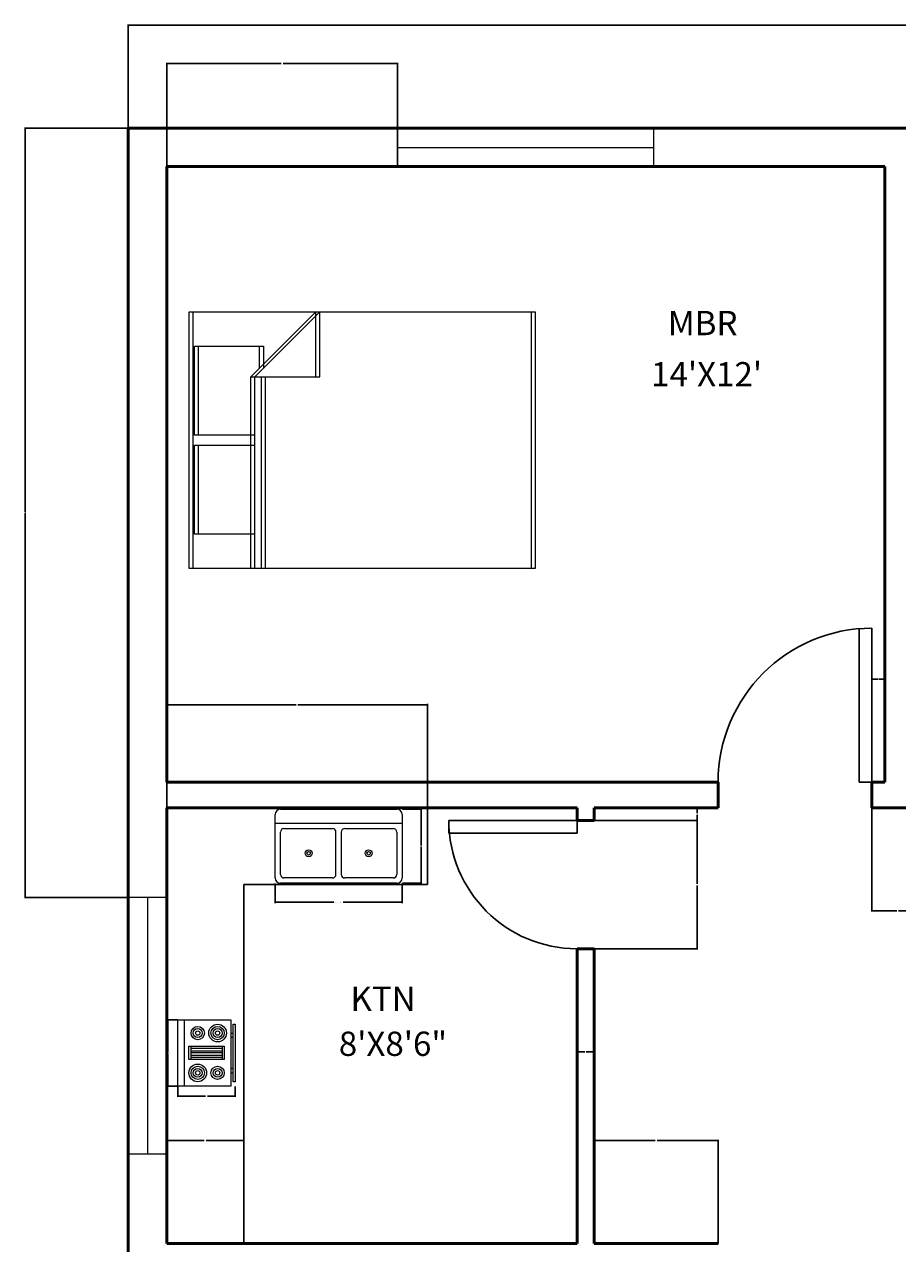
# Model space of a CAD drawing. Units: inches. Extents: x 66 to 499, y 601 to 1111.
# Tile 3 of 4: x 66 to 271, y 826 to 1111. Entities that reach past the tile are written whole.
import ezdxf

# ---------------------------------------------------------------- set-up
doc = ezdxf.new("R2010")
doc.units = ezdxf.units.IN
for name, color, linetype, lineweight in [('A-ANNO-DIMS', 2, 'Continuous', 18), ('A-AREA-IDEN', 7, 'Continuous', 18), ('A-DOOR', 3, 'Continuous', 25), ('A-EQPM', 8, 'Continuous', 18), ('A-FLOR-CASE', 9, 'Continuous', 25), ('A-FLOR-FIXT', 9, 'Continuous', 18), ('A-FURN', 8, 'Continuous', 18), ('A-GLAZ', 4, 'Continuous', 18), ('A-WALL', 7, 'Continuous', 50)]:
    doc.layers.add(name, color=color, linetype=linetype, lineweight=lineweight)
doc.styles.get("Standard").update_dxf_attribs({"font": 'arial.ttf'})
doc.dimstyles.get("Standard").update_dxf_attribs({"dimtxt": 0.18, "dimasz": 0.18, "dimexe": 0.18, "dimexo": 0.0625, "dimgap": 0.09, "dimtad": 0, "dimtih": 1, "dimtoh": 1, "dimdec": 4, "dimzin": 0, "dimdsep": 46, "dimtxsty": 'Standard', "dimcen": 0.09, "dimadec": 0, "dimazin": 0, "dimtfac": 1, "dimtdec": 4, "dimtofl": 0, "dimtmove": 0, "dimatfit": 3, "dimfxl": 1, "dimtolj": 1, "dimtzin": 0, "dimarcsym": 0})

# ---------------------------------------------------------------- blocks, each defined once
blk = doc.blocks.new('Sink-double - 36 in top')
for p, q in [((-18, -4), (18, -4)), ((-0.75, -18.5), (-0.75, -6.5)), ((0.75, -6.5), (0.75, -18.5))]:
    blk.add_line(p, q)
for points in [[(-16.5, 0), (16.5, 0)], [(-18, -19.5), (-18, -1.5)], [(18, -1.5), (18, -19.5)], [(-16.5, -18.5), (-16.5, -6.5)], [(-15.5, -5.5), (-1.75, -5.5)], [(1.75, -5.5), (15.5, -5.5)], [(16.5, -6.5), (16.5, -18.5)], [(-1.75, -19.5), (-15.5, -19.5)], [(15.5, -19.5), (1.75, -19.5)], [(16.5, -21), (-16.5, -21)]]:
    blk.add_lwpolyline(points)
for centre, radius in [((-8.5, -12.5), 1), ((-8.5, -12.5), 0.5), ((8.5, -12.5), 1), ((8.5, -12.5), 0.5)]:
    blk.add_circle(centre, radius)
for centre, radius, start, end in [((-16.5, -1.5), 1.5, 90, 180), ((16.5, -1.5), 1.5, 0, 90), ((-15.5, -6.5), 1, 90, 180), ((-1.75, -6.5), 1, 0, 90), ((1.75, -6.5), 1, 90, 180), ((15.5, -6.5), 1, 0, 90), ((-16.5, -19.5), 1.5, 180, 270), ((-15.5, -18.5), 1, 180, 270), ((-1.75, -18.5), 1, 270, 0), ((1.75, -18.5), 1, 180, 270), ((15.5, -18.5), 1, 270, 0), ((16.5, -19.5), 1.5, 270, 0)]:
    blk.add_arc(centre, radius, start, end)
blk = doc.blocks.new('Range-Oven - 30 in top')
for p, q in [((0, -3), (30, -3)), ((12, -6), (18, -6)), ((13, -20), (13, -6)), ((14, -6), (14, -20)), ((15, -20), (15, -6)), ((16, -6), (16, -20)), ((17, -20), (17, -6)), ((18, -20), (12, -20)), ((6, -24), (6, -25)), ((8, -25), (8, -24)), ((22, -25), (22, -24)), ((24, -24), (24, -25))]:
    blk.add_line(p, q)
for points in [[(0, -24), (0, 0), (30, 0), (30, -24)], [(12, -21), (12, -5), (18, -5), (18, -21)], [(2, -26), (2, -25), (28, -25), (28, -26)]]:
    blk.add_lwpolyline(points, close=True)
for centre, radius in [((6, -9), 4), ((6, -9), 3), ((6, -9), 2), ((6, -9), 1), ((24, -9), 3), ((24, -9), 2), ((24, -9), 1), ((6, -18), 3), ((6, -18), 2), ((24, -18), 4), ((24, -18), 3), ((24, -18), 2), ((6, -18), 1), ((24, -18), 1)]:
    blk.add_circle(centre, radius)
blk = doc.blocks.new('Bed - Queen')
for p, q in [((0, -80.00003), (0, 0)), ((0, 0), (59.99999, 0)), ((59.99999, 0), (59.99999, -80.00003)), ((7.99999, -1.2), (28.79998, -1.2)), ((7.99999, -14.4), (7.99999, -1.2)), ((28.79998, -1.2), (28.79998, -14.4)), ((31.19999, -1.2), (51.99999, -1.2)), ((31.19999, -14.4), (31.19999, -1.2)), ((51.99999, -1.2), (51.99999, -16.4)), ((0, -14.4), (44.8, -14.4)), ((44.8, -16.8), (0, -16.8)), ((59.99999, -29.6), (44.8, -14.4)), ((44.8, -14.4), (44.8, -29.6)), ((51.99999, -16.4), (46.79936, -16.4)), ((44.8, -29.6), (59.99999, -29.6)), ((59.99999, -80.00003), (0, -80.00003))]:
    blk.add_line(p, q)
blk = doc.blocks.new('DOOR-SWING-36IN')
for p, q in [((0, 36), (0, 0)), ((3, 36), (3, 0)), ((0, 0), (3, 0))]:
    blk.add_line(p, q)
blk.add_arc((0, 0), 36, 0, 90)
blk = doc.blocks.new('WIN-60IN')
for p, q in [((60, 9), (0, 9)), ((0, 9), (0, 0)), ((60, 0), (60, 9)), ((0, 4.5), (60, 4.5)), ((0, 0), (60, 0))]:
    blk.add_line(p, q)
blk = doc.blocks.new('*D38')
at = {"layer": 'A-ANNO-DIMS', "color": 0, "lineweight": -2, "transparency": 16777216}
for p, q in [((124.94, 910.26), (124.94, 905.69)), ((154.65, 910.26), (154.65, 905.69)), ((125.12, 905.87), (138.7, 905.87)), ((154.47, 905.87), (140.89, 905.87))]:
    blk.add_line(p, q, dxfattribs=at)
at = {"layer": 'A-ANNO-DIMS', "color": 0, "transparency": 16777216}
for points in [[(125.12, 905.9), (125.12, 905.84), (124.94, 905.87)], [(154.47, 905.9), (154.47, 905.84), (154.65, 905.87)]]:
    blk.add_solid(points, dxfattribs=at)
at = {"layer": 'Defpoints', "color": 0, "transparency": 16777216}
for p in [(124.94, 910.33), (154.65, 910.33), (154.65, 905.87)]:
    blk.add_point(p, dxfattribs=at)
at = {"layer": 'A-ANNO-DIMS', "color": 0, "transparency": 16777216, "insert": (139.79, 905.87), "char_height": 0.18, "attachment_point": 5}
blk.add_mtext('\\A1;DOUBLE SINK 30', dxfattribs=at)
blk = doc.blocks.new('*D39')
at = {"layer": 'A-ANNO-DIMS', "color": 0, "lineweight": -2, "transparency": 16777216}
for p, q in [((154.71, 927.65), (159.28, 927.65)), ((159.1, 927.47), (159.1, 919.17)), ((159.1, 910.51), (159.1, 918.81)), ((154.71, 910.33), (159.28, 910.33))]:
    blk.add_line(p, q, dxfattribs=at)
at = {"layer": 'A-ANNO-DIMS', "color": 0, "transparency": 16777216}
for points in [[(159.07, 927.47), (159.13, 927.47), (159.1, 927.65)], [(159.07, 910.51), (159.13, 910.51), (159.1, 910.33)]]:
    blk.add_solid(points, dxfattribs=at)
at = {"layer": 'Defpoints', "color": 0, "transparency": 16777216}
for p in [(154.65, 927.65), (159.1, 927.65), (154.65, 910.33)]:
    blk.add_point(p, dxfattribs=at)
at = {"layer": 'A-ANNO-DIMS', "color": 0, "transparency": 16777216, "insert": (159.1, 918.99), "char_height": 0.18, "attachment_point": 5}
blk.add_mtext('\\A1;17', dxfattribs=at)
blk = doc.blocks.new('*D40')
at = {"layer": 'A-ANNO-DIMS', "color": 0, "lineweight": -2, "transparency": 16777216}
for p, q in [((102.1, 878.38), (99.66, 878.38)), ((99.84, 878.2), (99.84, 870.8)), ((99.84, 863.03), (99.84, 870.43)), ((102.1, 862.85), (99.66, 862.85))]:
    blk.add_line(p, q, dxfattribs=at)
at = {"layer": 'A-ANNO-DIMS', "color": 0, "transparency": 16777216}
for points in [[(99.81, 878.2), (99.87, 878.2), (99.84, 878.38)], [(99.81, 863.03), (99.87, 863.03), (99.84, 862.85)]]:
    blk.add_solid(points, dxfattribs=at)
at = {"layer": 'Defpoints', "color": 0, "transparency": 16777216}
for p in [(99.84, 878.38), (102.17, 878.38), (102.17, 862.85)]:
    blk.add_point(p, dxfattribs=at)
at = {"layer": 'A-ANNO-DIMS', "color": 0, "transparency": 16777216, "insert": (99.84, 870.62), "char_height": 0.18, "attachment_point": 5}
blk.add_mtext('\\A1;RANGE 16', dxfattribs=at)
blk = doc.blocks.new('*D41')
at = {"layer": 'A-ANNO-DIMS', "color": 0, "lineweight": -2, "transparency": 16777216}
for p, q in [((102.17, 862.79), (102.17, 860.35)), ((115.62, 862.79), (115.62, 860.35)), ((102.35, 860.53), (108.68, 860.53)), ((115.44, 860.53), (109.1, 860.53))]:
    blk.add_line(p, q, dxfattribs=at)
at = {"layer": 'A-ANNO-DIMS', "color": 0, "transparency": 16777216}
for points in [[(102.35, 860.56), (102.35, 860.5), (102.17, 860.53)], [(115.44, 860.56), (115.44, 860.5), (115.62, 860.53)]]:
    blk.add_solid(points, dxfattribs=at)
at = {"layer": 'Defpoints', "color": 0, "transparency": 16777216}
for p in [(102.17, 862.85), (115.62, 862.85), (102.17, 860.53)]:
    blk.add_point(p, dxfattribs=at)
at = {"layer": 'A-ANNO-DIMS', "color": 0, "transparency": 16777216, "insert": (108.89, 860.53), "char_height": 0.18, "attachment_point": 5}
blk.add_mtext('\\A1;13', dxfattribs=at)
blk = doc.blocks.new('*D42')
at = {"layer": 'A-ANNO-DIMS', "color": 0, "lineweight": -2, "transparency": 16777216}
for p, q in [((90.58, 1087.07), (90.58, 1111.28)), ((90.76, 1111.1), (282.29, 1111.1)), ((474.4, 1111.1), (282.86, 1111.1)), ((474.58, 1087.07), (474.58, 1111.28))]:
    blk.add_line(p, q, dxfattribs=at)
at = {"layer": 'A-ANNO-DIMS', "color": 0, "transparency": 16777216}
for points in [[(90.76, 1111.13), (90.76, 1111.07), (90.58, 1111.1)], [(474.4, 1111.13), (474.4, 1111.07), (474.58, 1111.1)]]:
    blk.add_solid(points, dxfattribs=at)
at = {"layer": 'Defpoints', "color": 0, "transparency": 16777216}
for p in [(474.58, 1111.1), (90.58, 1087), (474.58, 1087)]:
    blk.add_point(p, dxfattribs=at)
at = {"layer": 'A-ANNO-DIMS', "color": 0, "transparency": 16777216, "insert": (282.58, 1111.1), "char_height": 0.18, "attachment_point": 5}
blk.add_mtext('\\A1;384', dxfattribs=at)
blk = doc.blocks.new('*D44')
at = {"layer": 'A-ANNO-DIMS', "color": 0, "lineweight": -2, "transparency": 16777216}
for p, q in [((99.58, 1078.07), (99.58, 1102.28)), ((99.76, 1102.1), (126.36, 1102.1)), ((153.4, 1102.1), (126.79, 1102.1)), ((153.58, 1078.07), (153.58, 1102.28))]:
    blk.add_line(p, q, dxfattribs=at)
at = {"layer": 'A-ANNO-DIMS', "color": 0, "transparency": 16777216}
for points in [[(99.76, 1102.13), (99.76, 1102.07), (99.58, 1102.1)], [(153.4, 1102.13), (153.4, 1102.07), (153.58, 1102.1)]]:
    blk.add_solid(points, dxfattribs=at)
at = {"layer": 'Defpoints', "color": 0, "transparency": 16777216}
for p in [(153.58, 1102.1), (99.58, 1078), (153.58, 1078)]:
    blk.add_point(p, dxfattribs=at)
at = {"layer": 'A-ANNO-DIMS', "color": 0, "transparency": 16777216, "insert": (126.58, 1102.1), "char_height": 0.18, "attachment_point": 5}
blk.add_mtext('\\A1;54', dxfattribs=at)
blk = doc.blocks.new('*D48')
at = {"layer": 'A-ANNO-DIMS', "color": 0, "lineweight": -2, "transparency": 16777216}
for p, q in [((90.51, 1087), (66.3, 1087)), ((66.48, 1086.82), (66.48, 997.19)), ((66.48, 907.18), (66.48, 996.82)), ((90.51, 907), (66.3, 907))]:
    blk.add_line(p, q, dxfattribs=at)
at = {"layer": 'A-ANNO-DIMS', "color": 0, "transparency": 16777216}
for points in [[(66.45, 1086.82), (66.51, 1086.82), (66.48, 1087)], [(66.45, 907.18), (66.51, 907.18), (66.48, 907)]]:
    blk.add_solid(points, dxfattribs=at)
at = {"layer": 'Defpoints', "color": 0, "transparency": 16777216}
for p in [(90.58, 1087), (66.48, 907), (90.58, 907)]:
    blk.add_point(p, dxfattribs=at)
at = {"layer": 'A-ANNO-DIMS', "color": 0, "transparency": 16777216, "insert": (66.48, 997), "char_height": 0.18, "attachment_point": 5}
blk.add_mtext('\\A1;180', dxfattribs=at)
blk = doc.blocks.new('*D56')
at = {"layer": 'A-ANNO-DIMS', "color": 0, "lineweight": -2, "transparency": 16777216}
for p, q in [((199.64, 925), (223.86, 925)), ((223.68, 924.82), (223.68, 910.19)), ((223.68, 895.18), (223.68, 909.82)), ((199.64, 895), (223.86, 895))]:
    blk.add_line(p, q, dxfattribs=at)
at = {"layer": 'A-ANNO-DIMS', "color": 0, "transparency": 16777216}
for points in [[(223.65, 924.82), (223.71, 924.82), (223.68, 925)], [(223.65, 895.18), (223.71, 895.18), (223.68, 895)]]:
    blk.add_solid(points, dxfattribs=at)
at = {"layer": 'Defpoints', "color": 0, "transparency": 16777216}
for p in [(199.58, 925), (199.58, 895), (223.68, 895)]:
    blk.add_point(p, dxfattribs=at)
at = {"layer": 'A-ANNO-DIMS', "color": 0, "transparency": 16777216, "insert": (223.68, 910), "char_height": 0.18, "attachment_point": 5}
blk.add_mtext('\\A1;30', dxfattribs=at)
blk = doc.blocks.new('*D57')
at = {"layer": 'A-ANNO-DIMS', "color": 0, "lineweight": -2, "transparency": 16777216}
for p, q in [((199.58, 826.07), (199.58, 850.28)), ((228.58, 826.07), (228.58, 850.28)), ((199.76, 850.1), (213.86, 850.1)), ((228.4, 850.1), (214.3, 850.1))]:
    blk.add_line(p, q, dxfattribs=at)
at = {"layer": 'A-ANNO-DIMS', "color": 0, "transparency": 16777216}
for points in [[(199.76, 850.13), (199.76, 850.07), (199.58, 850.1)], [(228.4, 850.13), (228.4, 850.07), (228.58, 850.1)]]:
    blk.add_solid(points, dxfattribs=at)
at = {"layer": 'Defpoints', "color": 0, "transparency": 16777216}
for p in [(228.58, 850.1), (199.58, 826), (228.58, 826)]:
    blk.add_point(p, dxfattribs=at)
at = {"layer": 'A-ANNO-DIMS', "color": 0, "transparency": 16777216, "insert": (214.08, 850.1), "char_height": 0.18, "attachment_point": 5}
blk.add_mtext('\\A1;29', dxfattribs=at)
blk = doc.blocks.new('*D58')
at = {"layer": 'A-ANNO-DIMS', "color": 0, "lineweight": -2, "transparency": 16777216}
for p, q in [((264.58, 927.94), (264.58, 903.72)), ((276.58, 927.94), (276.58, 903.72)), ((264.76, 903.9), (270.37, 903.9)), ((276.4, 903.9), (270.79, 903.9))]:
    blk.add_line(p, q, dxfattribs=at)
at = {"layer": 'A-ANNO-DIMS', "color": 0, "transparency": 16777216}
for points in [[(264.76, 903.93), (264.76, 903.87), (264.58, 903.9)], [(276.4, 903.93), (276.4, 903.87), (276.58, 903.9)]]:
    blk.add_solid(points, dxfattribs=at)
at = {"layer": 'Defpoints', "color": 0, "transparency": 16777216}
for p in [(264.58, 928), (276.58, 928), (264.58, 903.9)]:
    blk.add_point(p, dxfattribs=at)
at = {"layer": 'A-ANNO-DIMS', "color": 0, "transparency": 16777216, "insert": (270.58, 903.9), "char_height": 0.18, "attachment_point": 5}
blk.add_mtext('\\A1;12', dxfattribs=at)
blk = doc.blocks.new('*D59')
at = {"layer": 'A-ANNO-DIMS', "color": 0, "lineweight": -2, "transparency": 16777216}
for p, q in [((99.58, 826.07), (99.58, 850.28)), ((117.58, 826.07), (117.58, 850.28)), ((99.76, 850.1), (108.37, 850.1)), ((117.4, 850.1), (108.79, 850.1))]:
    blk.add_line(p, q, dxfattribs=at)
at = {"layer": 'A-ANNO-DIMS', "color": 0, "transparency": 16777216}
for points in [[(99.76, 850.13), (99.76, 850.07), (99.58, 850.1)], [(117.4, 850.13), (117.4, 850.07), (117.58, 850.1)]]:
    blk.add_solid(points, dxfattribs=at)
at = {"layer": 'Defpoints', "color": 0, "transparency": 16777216}
for p in [(117.58, 850.1), (99.58, 826), (117.58, 826)]:
    blk.add_point(p, dxfattribs=at)
at = {"layer": 'A-ANNO-DIMS', "color": 0, "transparency": 16777216, "insert": (108.58, 850.1), "char_height": 0.18, "attachment_point": 5}
blk.add_mtext('\\A1;18', dxfattribs=at)
blk = doc.blocks.new('*D60')
at = {"layer": 'A-ANNO-DIMS', "color": 0, "lineweight": -2, "transparency": 16777216}
for p, q in [((99.58, 928.07), (99.58, 952.28)), ((99.76, 952.1), (129.87, 952.1)), ((160.4, 952.1), (130.28, 952.1)), ((160.58, 928.07), (160.58, 952.28))]:
    blk.add_line(p, q, dxfattribs=at)
at = {"layer": 'A-ANNO-DIMS', "color": 0, "transparency": 16777216}
for points in [[(99.76, 952.13), (99.76, 952.07), (99.58, 952.1)], [(160.4, 952.13), (160.4, 952.07), (160.58, 952.1)]]:
    blk.add_solid(points, dxfattribs=at)
at = {"layer": 'Defpoints', "color": 0, "transparency": 16777216}
for p in [(160.58, 952.1), (99.58, 928), (160.58, 928)]:
    blk.add_point(p, dxfattribs=at)
at = {"layer": 'A-ANNO-DIMS', "color": 0, "transparency": 16777216, "insert": (130.08, 952.1), "char_height": 0.18, "attachment_point": 5}
blk.add_mtext('\\A1;61', dxfattribs=at)
blk = doc.blocks.new('*D61')
at = {"layer": 'A-ANNO-DIMS', "color": 0, "lineweight": -2, "transparency": 16777216}
for p, q in [((195.58, 894.94), (195.58, 870.72)), ((199.58, 894.94), (199.58, 870.72)), ((195.76, 870.9), (197.42, 870.9)), ((199.4, 870.9), (197.73, 870.9))]:
    blk.add_line(p, q, dxfattribs=at)
at = {"layer": 'A-ANNO-DIMS', "color": 0, "transparency": 16777216}
for points in [[(195.76, 870.93), (195.76, 870.87), (195.58, 870.9)], [(199.4, 870.93), (199.4, 870.87), (199.58, 870.9)]]:
    blk.add_solid(points, dxfattribs=at)
at = {"layer": 'Defpoints', "color": 0, "transparency": 16777216}
for p in [(195.58, 895), (199.58, 895), (195.58, 870.9)]:
    blk.add_point(p, dxfattribs=at)
at = {"layer": 'A-ANNO-DIMS', "color": 0, "transparency": 16777216, "insert": (197.58, 870.9), "char_height": 0.18, "attachment_point": 5}
blk.add_mtext('\\A1;4', dxfattribs=at)
blk = doc.blocks.new('*D65')
at = {"layer": 'A-ANNO-DIMS', "color": 0, "lineweight": -2, "transparency": 16777216}
for p, q in [((264.58, 934.07), (264.58, 958.28)), ((264.76, 958.1), (265.93, 958.1)), ((267.4, 958.1), (266.22, 958.1)), ((267.58, 934.07), (267.58, 958.28))]:
    blk.add_line(p, q, dxfattribs=at)
at = {"layer": 'A-ANNO-DIMS', "color": 0, "transparency": 16777216}
for points in [[(264.76, 958.13), (264.76, 958.07), (264.58, 958.1)], [(267.4, 958.13), (267.4, 958.07), (267.58, 958.1)]]:
    blk.add_solid(points, dxfattribs=at)
at = {"layer": 'Defpoints', "color": 0, "transparency": 16777216}
for p in [(267.58, 958.1), (264.58, 934), (267.58, 934)]:
    blk.add_point(p, dxfattribs=at)
at = {"layer": 'A-ANNO-DIMS', "color": 0, "transparency": 16777216, "insert": (266.08, 958.1), "char_height": 0.18, "attachment_point": 5}
blk.add_mtext('\\A1;3', dxfattribs=at)
blk = doc.blocks.new('*D66')
at = {"layer": 'A-ANNO-DIMS', "color": 0, "lineweight": -2, "transparency": 16777216}
for p, q in [((199.64, 928), (223.86, 928)), ((223.68, 927.82), (223.68, 926.69)), ((199.64, 925), (223.86, 925)), ((223.68, 925.18), (223.68, 926.32))]:
    blk.add_line(p, q, dxfattribs=at)
at = {"layer": 'A-ANNO-DIMS', "color": 0, "transparency": 16777216}
for points in [[(223.65, 927.82), (223.71, 927.82), (223.68, 928)], [(223.65, 925.18), (223.71, 925.18), (223.68, 925)]]:
    blk.add_solid(points, dxfattribs=at)
at = {"layer": 'Defpoints', "color": 0, "transparency": 16777216}
for p in [(199.58, 928), (199.58, 925), (223.68, 925)]:
    blk.add_point(p, dxfattribs=at)
at = {"layer": 'A-ANNO-DIMS', "color": 0, "transparency": 16777216, "insert": (223.68, 926.5), "char_height": 0.18, "attachment_point": 5}
blk.add_mtext('\\A1;3', dxfattribs=at)

msp = doc.modelspace()

# ---------------------------------------------------------------- linework, layer by layer
at = {"layer": 'A-DOOR'}
for p, q in [((165.5757, 925.0042), (195.5757, 925.0042)), ((165.5757, 925.0042), (165.5757, 922.0042)), ((195.5757, 925.0042), (195.5706, 922.0042)), ((165.5757, 922.0042), (195.5757, 922.0042))]:
    msp.add_line(p, q, dxfattribs=at)
msp.add_arc((195.5757, 925.0042), 30, 180, 269.902326, dxfattribs=at)
at = {"layer": 'A-FLOR-CASE'}
for p, q in [((160.5757, 928.0042), (160.5757, 910.0042)), ((117.5757, 910.0042), (117.5757, 826.0042)), ((160.5757, 910.0042), (117.5757, 910.0042))]:
    msp.add_line(p, q, dxfattribs=at)
at = {"layer": 'A-WALL'}
for p, q in [((99.5757, 1078.0042), (99.5757, 934.0042)), ((267.5757, 1078.0042), (99.5757, 1078.0042)), ((267.5757, 1078.0042), (267.5757, 934.0042)), ((228.5757, 934.0042), (99.5757, 934.0042)), ((228.5757, 934.0042), (228.5757, 928.0042)), ((267.5757, 934.0042), (264.5757, 934.0042)), ((264.5757, 934.0042), (264.5757, 928.0042)), ((195.5757, 928.0042), (99.5757, 928.0042)), ((99.5757, 928.0042), (99.5757, 826.0042)), ((195.5757, 928.0042), (195.5757, 925.0042)), ((199.5757, 928.0042), (199.5757, 925.0042)), ((228.5757, 928.0042), (199.5757, 928.0042)), ((267.5757, 928.0042), (264.5757, 928.0042)), ((267.5757, 928.0042), (273.5757, 928.0042)), ((199.5757, 925.0042), (195.5757, 925.0042)), ((199.5757, 895.0042), (195.5757, 895.0042)), ((195.5757, 895.0042), (195.5757, 826.0042)), ((199.5757, 895.0042), (199.5757, 826.0042)), ((195.5757, 826.0042), (99.5757, 826.0042)), ((228.5757, 826.0042), (199.5757, 826.0042))]:
    msp.add_line(p, q, dxfattribs=at)
msp.add_lwpolyline([(90.5757, 625.0042), (474.5757, 625.0042), (474.5757, 1087.0042), (90.5757, 1087.0042)], close=True, dxfattribs=at)

# ---------------------------------------------------------------- block references
at = {"layer": 'A-DOOR', "extrusion": (0, 0, -1), "zscale": -1}
msp.add_blockref('DOOR-SWING-36IN', (-264.5757, 934.0042), dxfattribs=at)
at = {"layer": 'A-EQPM', "xscale": 0.5174613357638611, "yscale": 0.5174613357638611, "zscale": 0.5174613357638611, "rotation": 90}
msp.add_blockref('Range-Oven - 30 in top', (102.1657, 862.8548), dxfattribs=at)
at = {"layer": 'A-FLOR-FIXT', "xscale": 0.8250810528887459, "yscale": 0.8250810528887459, "zscale": 0.8250810528887459}
msp.add_blockref('Sink-double - 36 in top', (139.7936, 927.6523), dxfattribs=at)
at = {"layer": 'A-FURN', "rotation": 90}
for p in [(104.8378, 983.9965), (105.7788, 983.9965)]:
    msp.add_blockref('Bed - Queen', p, dxfattribs=at)
at = {"layer": 'A-GLAZ'}
msp.add_blockref('WIN-60IN', (153.5757, 1078.0042), dxfattribs=at)
at = {"layer": 'A-GLAZ', "rotation": 270.0000000000001}
msp.add_blockref('WIN-60IN', (90.5757, 907.0042), dxfattribs=at)

# ---------------------------------------------------------------- texts
at = {"layer": 'A-AREA-IDEN', "char_height": 5.6821, "attachment_point": 1}
for s, insert in [('MBR', (216.8061, 1044.2449)), ("14'X12'", (212.9051, 1032.2727)), ('KTN', (142.557, 886.1525)), ('8\'X8\'6"', (139.8366, 875.604))]:
    msp.add_mtext_dynamic_manual_height_columns(s, width=58.656418, gutter_width=28.4105, heights=[0], dxfattribs=dict(at, insert=insert))

# ---------------------------------------------------------------- dimensions: what is measured, and where the dimension line sits
at = {"layer": 'A-ANNO-DIMS'}
for base, p1, p2, picture, middle in [((474.5757, 1111.1042), (90.5757, 1087.0042), (474.5757, 1087.0042), '*D42', (282.5757, 1111.1042)), ((267.5757, 958.1042), (264.5757, 934.0042), (267.5757, 934.0042), '*D65', (266.0757, 958.1042)), ((160.5757, 952.1042), (99.5757, 928.0042), (160.5757, 928.0042), '*D60', (130.0757, 952.1042)), ((117.5757, 850.1042), (99.5757, 826.0042), (117.5757, 826.0042), '*D59', (108.5757, 850.1042)), ((228.5757, 850.1042), (199.5757, 826.0042), (228.5757, 826.0042), '*D57', (214.0757, 850.1042))]:
    dim = msp.add_linear_dim(base=base, p1=p1, p2=p2, dimstyle='Standard', override={"dimdec": 0, "dimlfac": 1, "dimrnd": 0, "dimzin": 0, "dimdsep": 46, "dimlunit": 2}, dxfattribs=at)
    dim.commit()
    dim.dimension.update_dxf_attribs({"geometry": picture, "text_midpoint": middle})
for base, p1, p2, angle, picture, middle in [((153.5757, 1102.1042), (99.5757, 1078.0042), (153.5757, 1078.0042), 0, '*D44', (126.5757, 1102.1042)), ((66.4757, 907.0042), (90.5757, 1087.0042), (90.5757, 907.0042), 90, '*D48', (66.4757, 997.0042)), ((159.1005, 927.6523), (154.6451, 910.3256), (154.6451, 927.6523), 90, '*D39', (159.1005, 918.9889)), ((223.6757, 925.0042), (199.5757, 928.0042), (199.5757, 925.0042), 270, '*D66', (223.6757, 926.5042)), ((264.5757, 903.9042), (276.5757, 928.0042), (264.5757, 928.0042), 180, '*D58', (270.5757, 903.9042)), ((223.6757, 895.0042), (199.5757, 925.0042), (199.5757, 895.0042), 270, '*D56', (223.6757, 910.0042)), ((195.5757, 870.9042), (199.5757, 895.0042), (195.5757, 895.0042), 180, '*D61', (197.5757, 870.9042)), ((102.1657, 860.5262), (115.6197, 862.8548), (102.1657, 862.8548), 180, '*D41', (108.8927, 860.5262))]:
    dim = msp.add_linear_dim(base=base, p1=p1, p2=p2, angle=angle, dimstyle='Standard', override={"dimdec": 0, "dimlfac": 1, "dimrnd": 0, "dimzin": 0, "dimdsep": 46, "dimlunit": 2}, dxfattribs=at)
    dim.commit()
    dim.dimension.update_dxf_attribs({"geometry": picture, "text_midpoint": middle})
dim = msp.add_linear_dim(base=(154.6451, 905.8701), p1=(124.9422, 910.3256), p2=(154.6451, 910.3256), text='DOUBLE SINK <>', dimstyle='Standard', override={"dimdec": 0, "dimlfac": 1, "dimrnd": 0, "dimzin": 0, "dimdsep": 46, "dimlunit": 2}, dxfattribs=at)
dim.commit()
dim.dimension.update_dxf_attribs({"geometry": '*D38', "text_midpoint": (139.7936, 905.8701)})
dim = msp.add_linear_dim(base=(99.8371, 878.3786), p1=(102.1657, 862.8548), p2=(102.1657, 878.3786), angle=90, text='RANGE <>', dimstyle='Standard', override={"dimdec": 0, "dimlfac": 1, "dimrnd": 0, "dimzin": 0, "dimdsep": 46, "dimlunit": 2}, dxfattribs=at)
dim.commit()
dim.dimension.update_dxf_attribs({"geometry": '*D40', "text_midpoint": (99.8371, 870.6167)})

doc.saveas('drawing.dxf')
